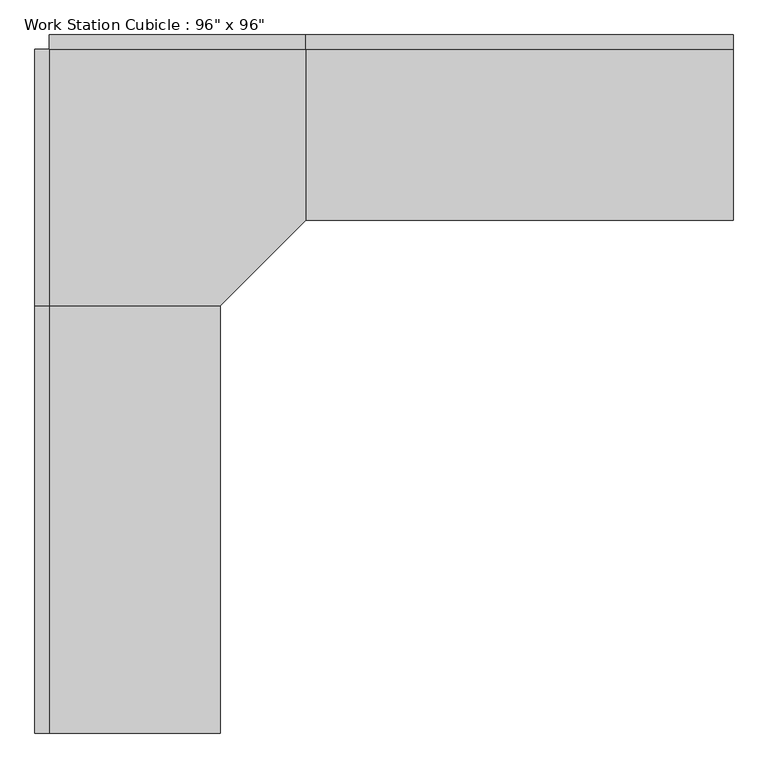
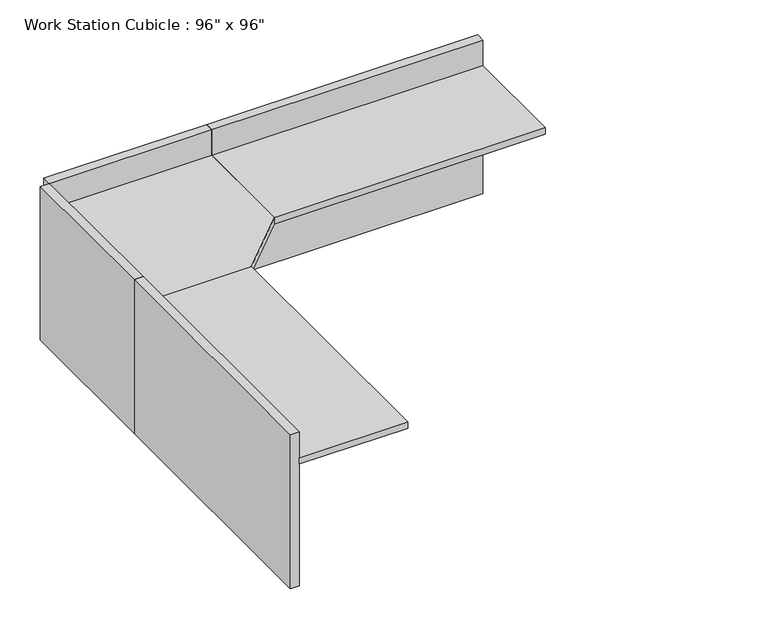
"""IFC4 building model written with IfcOpenShell, lengths in millimetres: furniture geometry."""

from ifc_helpers import new_model, si_unit, frame, origin, origin_with_axes, place, context, project, spatial, polyline, outline, extrude, source, transform, mapped, element, save


def furniture_125de5a1(model_context):
    return source(origin(), model_context, "Body", "SweptSolid", [
        extrude(outline(polyline([(-80.9317522, -545.8230076), (833.4682478, -545.8230076), (833.4682478, -1155.4230076), (528.6682478, -1460.2230076), (-80.9317522, -1460.2230076), (-80.9317522, -545.8230076)])), frame((0.0, 0.0, 723.9), z_axis=(0.0, 0.0, 1.0), x_axis=(1.0, 0.0, 0.0)), (0.0, 0.0, 1.0), 38.1),
        extrude(outline(polyline([(528.6682478, -2984.2230076), (-80.9317522, -2984.2230076), (-80.9317522, -1460.2230076), (528.6682478, -1460.2230076), (528.6682478, -2984.2230076)])), frame((0.0, 0.0, 723.9), z_axis=(0.0, 0.0, 1.0), x_axis=(1.0, 0.0, 0.0)), (0.0, 0.0, 1.0), 38.1),
        extrude(outline(polyline([(2357.4682478, -1155.4230076), (833.4682478, -1155.4230076), (833.4682478, -545.8230076), (2357.4682478, -545.8230076), (2357.4682478, -1155.4230076)])), frame((0.0, 0.0, 723.9), z_axis=(0.0, 0.0, 1.0), x_axis=(1.0, 0.0, 0.0)), (0.0, 0.0, 1.0), 38.1),
        extrude(outline(polyline([(2357.4682478, -545.8230076), (833.4682478, -545.8230076), (833.4682478, -495.0230076), (2357.4682478, -495.0230076), (2357.4682478, -545.8230076)])), origin_with_axes(), (0.0, 0.0, 1.0), 914.4),
        extrude(outline(polyline([(833.4682478, -545.8230076), (-80.9317522, -545.8230076), (-80.9317522, -495.0230076), (833.4682478, -495.0230076), (833.4682478, -545.8230076)])), origin_with_axes(), (0.0, 0.0, 1.0), 914.4),
        extrude(outline(polyline([(-80.9317522, -1460.2230076), (-131.7317522, -1460.2230076), (-131.7317522, -545.8230076), (-80.9317522, -545.8230076), (-80.9317522, -1460.2230076)])), origin_with_axes(), (0.0, 0.0, 1.0), 914.4),
        extrude(outline(polyline([(-80.9317522, -2984.2230076), (-131.7317522, -2984.2230076), (-131.7317522, -1460.2230076), (-80.9317522, -1460.2230076), (-80.9317522, -2984.2230076)])), origin_with_axes(), (0.0, 0.0, 1.0), 914.4),
    ])


if __name__ == "__main__":
    model = new_model("IFC4")
    model_context = context("Model", 3, world=origin())
    ifc_project = project(units=[si_unit("LENGTHUNIT", "METRE", prefix="MILLI")], contexts=[model_context])
    site = spatial("IfcSite", under=ifc_project)
    building = spatial("IfcBuilding", under=site)
    placement = place(None, origin())
    furniture_shape = furniture_125de5a1(model_context)
    element("IfcFurniture", 1, ObjectType="Work Station Cubicle : 96\" x 96\"", at=placement, inside=building, context=model_context, shape_type="MappedRepresentation", body=[
        mapped(furniture_shape, transform((0.0, 0.0, 0.0), x_axis=(1.0, 0.0, 0.0), y_axis=(0.0, 1.0, 0.0), z_axis=(0.0, 0.0, 1.0))),
    ])
    save(model, "model.ifc")

# Revit data of these elements
# Type "Work Station Cubicle : 96\" x 96\""
#   Assembly Code = "E2020"
#   Desktop Height = 2' - 6"
#   Desktop1 Width = 2' - 0"
#   Desktop2 Width = 2' - 0"
#   Panel Height = 3' - 0"
#   Panel1 Length = 5' - 0"
#   Panel2 Length = 5' - 0"
#   Cube Panel Material = Textile - Light Gray
#   Work Top Material = Laminate, Ivory, Matte
#   Default Elevation = 0
# Element 1 (IfcFurniture, "Work Station Cubicle : 96\" x 96\"")
#   Materials on its faces: "Textile - Light Gray", "Laminate, Ivory, Matte"
# Materials
#   "Textile - Light Gray": class "Fabric", colour RGB 204 204 204, transparency 0
#   "Laminate, Ivory, Matte": class "Plastic", colour RGB 247 247 239, transparency 0, Description = "Plastic Laminate - Ivory, Matte", Cost = 0
